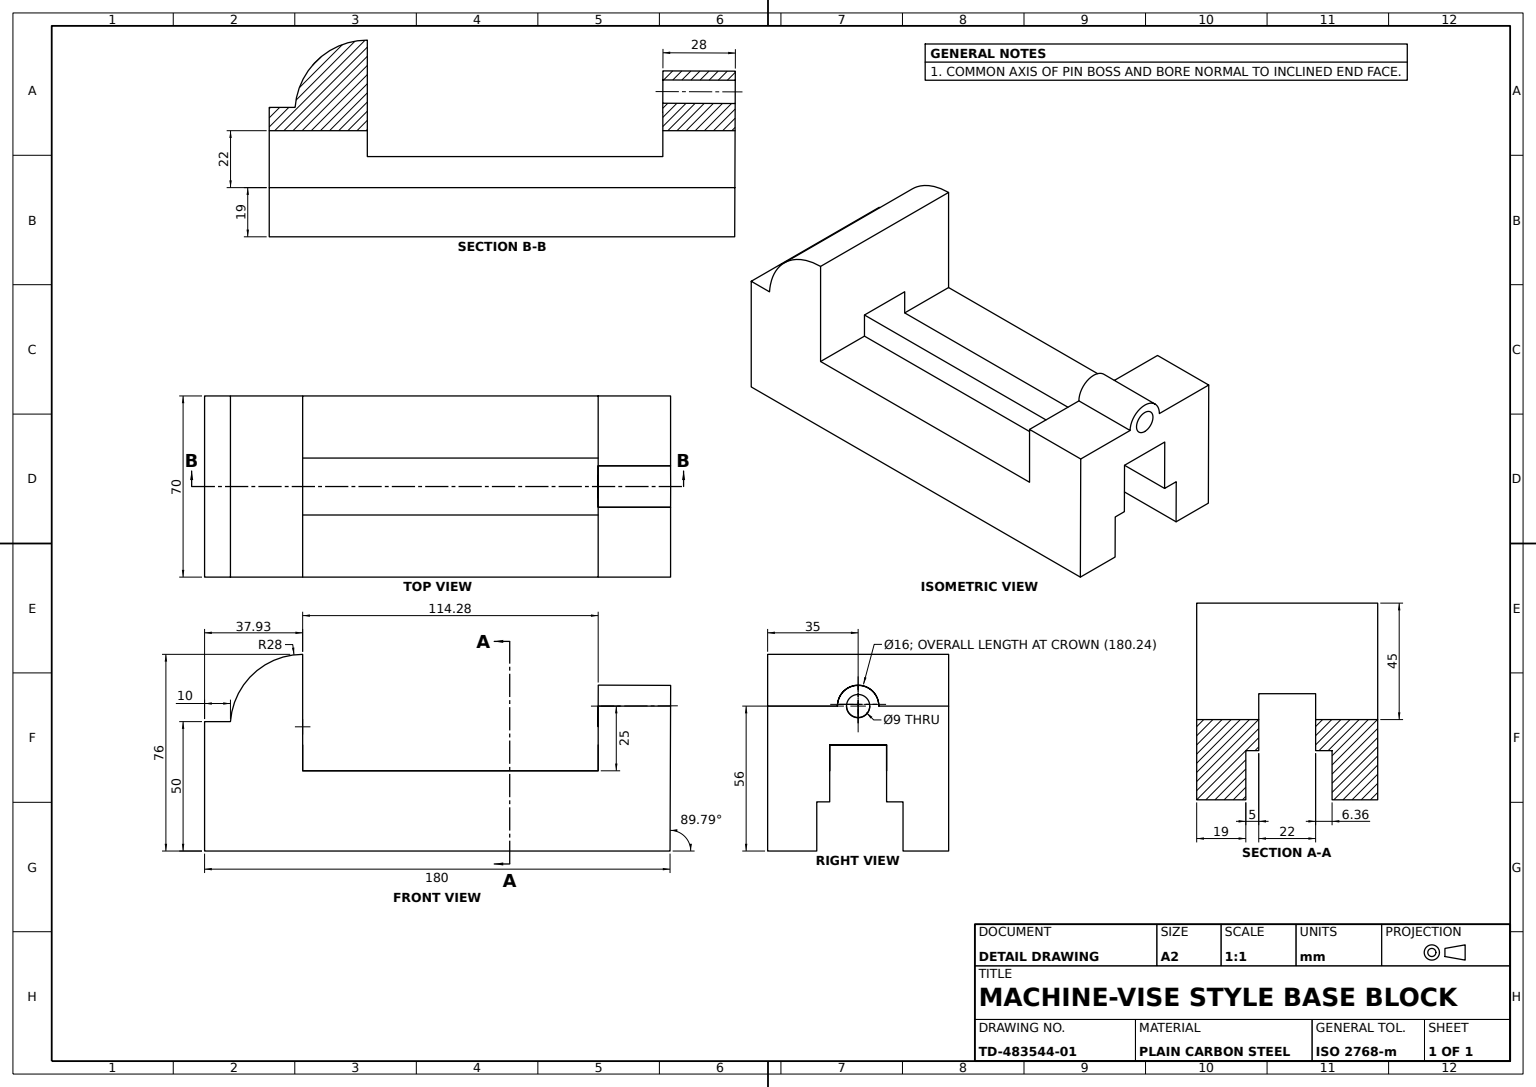
SolidWorks part; units mm, degrees
material "Plain Carbon Steel"
ref_plane "Front Plane" through (0, 0, 0) normal (0, 0, 1) x (1, 0, 0)
ref_plane "Top Plane" through (0, 0, 0) normal (0, 1, 0) x (1, 0, 0)
ref_plane "Right Plane" through (0, 0, 0) normal (1, 0, 0) x (0, 0, -1)
sketch "Base Profile Sketch" plane through (0, 0, 0) normal (0, 0, 1) x (1, 0, 0)
  line L0 (0, 0) -> (180, 0)
  line L1 (180, 0) -> (180.2091, 55.9996)
  line L2 (180.2091, 55.9996) -> (152.2091, 55.9996)
  line L3 (152.2091, 55.9996) -> (152.2091, 30.9996)
  line L4 (152.2091, 30.9996) -> (37.9285, 30.9996)
  line L5 (37.9285, 30.9996) -> (37.9285, 75.9996)
  line L6 (10, 50) -> (0, 50)
  line L7 (0, 50) -> (0, 0)
  arc A0 (37.9285, 75.9996) -> (10, 50) centre (37.9285, 47.9996) ccw
  dimension "D1" = 28
  dimension "D2" = 50
  dimension "D3" = 45
  dimension "D4" = 56
  dimension "D5" = 28
  dimension "D6" = 10
  dimension "D7" = 180
  dimension "D8" = 114.2806
  dimension "D9" = 25
extrude "Base Body" add sketch "Base Profile Sketch" against normal blind 70
sketch "Pin Boss Sketch" plane through (179.9975, -0.672, 0) normal (1, -0.0037, 0) x (0, 0, -1)
  line L0 (70, 56.672) -> (0, 56.672) construction
  circle A0 centre (35, 56.672) radius 8
  dimension "D1" = 16
extrude "Pin Boss" add sketch "Pin Boss Sketch" against normal blind 28
sketch "Pin Hole Sketch" plane through (179.9975, -0.672, 0) normal (1, -0.0037, 0) x (0, 0, -1)
  circle A0 centre (35, 56.672) radius 4.5
  dimension "D1" = 9
extrude "Pin Hole" cut sketch "Pin Hole Sketch" against normal blind 28
sketch "End Slot Sketch" plane through (0, 0, 0) normal (-1, 0, 0) x (0, 0, 1)
  line L0 (-52.3592, 0) -> (-52.3592, 19)
  line L1 (-70, 0) -> (0, 0) construction
  line L2 (-52.3592, 19) -> (-46, 19)
  line L3 (-46, 19) -> (-46, 41)
  line L4 (-46, 41) -> (-24, 41)
  line L5 (-24, 41) -> (-24, 19)
  line L6 (-24, 19) -> (-19, 19)
  line L7 (-19, 19) -> (-19, 0)
  line L8 (-19, 0) -> (-52.3592, 0)
  line L10 (-70, 50) -> (0, 50) construction
  point P18 (-35, 50)
  point P19 (-35, 41)
  dimension "D1" = 5
  dimension "D2" = 19
  dimension "D3" = 6.3592
  dimension "D4" = 22
  dimension "D5" = 19
  dimension "D6" = 19
extrude "End Slot Cut" cut sketch "End Slot Sketch" against normal through all
